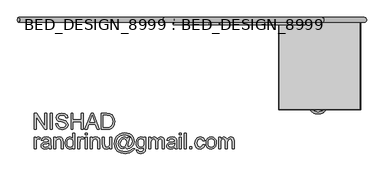
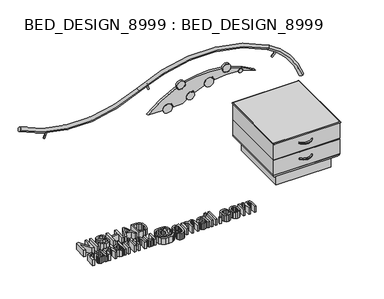
"""IFC4 building model written with IfcOpenShell, lengths in millimetres: furniture geometry, BED_DESIGN_8999 : BED_DESIGN_8999."""

from ifc_helpers import new_model, si_unit, point, frame, frame_2d, origin, origin_with_axes, place, context, project, spatial, polyline, circle_curve, ellipse_curve, trimmed, segment, composite_curve, outline, extrude, source, transform, mapped, element, save
from ifc_brep_helpers import plane_surface, cylinder_surface, revolved_surface, advanced_brep


def bed_design_8999_bed_design_8999_e911dec7(model_context):
    return source(origin(), model_context, "Body", "SolidModel", [
        advanced_brep(
        [(1204.2592917, 1919.1163159, 367.6654044), (1204.2592917, 1919.1163159, 242.6654044), (700.3023182, 1919.1163159, 242.6654044), (700.3023182, 1919.1163159, 367.6654044), (1129.2592917, 1844.1163159, 87.6654044), (1129.2592917, 1844.1163159, 367.6654044), (775.3023182, 1844.1163159, 367.6654044), (775.3023182, 1844.1163159, 87.6654044), (1204.2331329, 1919.0901571, 116.4128697), (1174.2592917, 1889.1163159, 87.6654044), (730.3023182, 1889.1163159, 87.6654044), (700.328477, 1919.0901571, 116.4128697), (1201.7592917, 1916.6163159, 118.9128697), (1201.7592917, 1916.6163159, 116.4128697), (702.8023182, 1916.6163159, 116.4128697), (702.8023182, 1916.6163159, 118.9128697), (1204.2592917, 1919.1163159, 237.6654044), (1204.2592917, 1919.1163159, 118.9128697), (700.3023182, 1919.1163159, 118.9128697), (700.3023182, 1919.1163159, 237.6654044), (1199.2592917, 1914.1163159, 242.6654044), (1199.2592917, 1914.1163159, 237.6654044), (705.3023182, 1914.1163159, 237.6654044), (705.3023182, 1914.1163159, 242.6654044), (700.3023182, 1379.1275792, 242.6654044), (700.3023182, 1379.1275792, 367.6654044), (775.3023182, 1454.1275792, 367.6654044), (775.3023182, 1454.1275792, 87.6654044), (730.3023182, 1409.1275792, 87.6654044), (700.328477, 1379.153738, 116.4128697), (702.8023182, 1381.6275792, 116.4128697), (702.8023182, 1381.6275792, 118.9128697), (700.3023182, 1379.1275792, 118.9128697), (700.3023182, 1379.1275792, 237.6654044), (705.3023182, 1384.1275792, 237.6654044), (705.3023182, 1384.1275792, 242.6654044), (1204.2592917, 1379.1275792, 242.6654044), (1204.2592917, 1379.1275792, 367.6654044), (1129.2592917, 1454.1275792, 367.6654044), (1129.2592917, 1454.1275792, 87.6654044), (1174.2592917, 1409.1275792, 87.6654044), (1204.2331329, 1379.153738, 116.4128697), (1201.7592917, 1381.6275792, 116.4128697), (1201.7592917, 1381.6275792, 118.9128697), (1204.2592917, 1379.1275792, 118.9128697), (1204.2592917, 1379.1275792, 237.6654044), (1199.2592917, 1384.1275792, 237.6654044), (1199.2592917, 1384.1275792, 242.6654044)],
        [
            (0, 1),
            (1, 2),
            (2, 3),
            (3, 0),
            (4, 5),
            (5, 6),
            (6, 7),
            (7, 4),
            (8, 9, ellipse_curve(frame((1174.2592917, 1889.1163159, 117.6654044), z_axis=(-0.7071067811865456, 0.7071067811865496, 0.0), x_axis=(0.7071067811865495, 0.7071067811865455, 0.0)), 42.4264069, 30.0)),
            (9, 10),
            (10, 11, ellipse_curve(frame((730.3023182, 1889.1163159, 117.6654044), z_axis=(0.7071067811865493, 0.7071067811865457, 0.0), x_axis=(0.7071067811865457, -0.7071067811865495, 0.0)), 42.4264069, 30.0)),
            (11, 8),
            (12, 13),
            (13, 14),
            (14, 15),
            (15, 12),
            (16, 17),
            (17, 18),
            (18, 19),
            (19, 16),
            (20, 21),
            (21, 22),
            (22, 23),
            (23, 20),
            (2, 24),
            (24, 25),
            (25, 3),
            (6, 26),
            (26, 27),
            (27, 7),
            (10, 28),
            (28, 29, ellipse_curve(frame((730.3023182, 1409.1275792, 117.6654044), z_axis=(-0.7071067811865457, 0.7071067811865495, 0.0), x_axis=(0.7071067811865495, 0.7071067811865456, 0.0)), 42.4264069, 30.0)),
            (29, 11),
            (14, 30),
            (30, 31),
            (31, 15),
            (18, 32),
            (32, 33),
            (33, 19),
            (22, 34),
            (34, 35),
            (35, 23),
            (24, 36),
            (36, 37),
            (37, 25),
            (26, 38),
            (38, 39),
            (39, 27),
            (28, 40),
            (40, 41, ellipse_curve(frame((1174.2592917, 1409.1275792, 117.6654044), z_axis=(-0.7071067811865496, -0.7071067811865455, 0.0), x_axis=(-0.7071067811865455, 0.7071067811865496, 0.0)), 42.4264069, 30.0)),
            (41, 29),
            (30, 42),
            (42, 43),
            (43, 31),
            (32, 44),
            (44, 45),
            (45, 33),
            (34, 46),
            (46, 47),
            (47, 35),
            (36, 1),
            (0, 37),
            (5, 38),
            (4, 39),
            (9, 40),
            (8, 41),
            (13, 42),
            (12, 43),
            (17, 44),
            (16, 45),
            (21, 46),
            (20, 47),
        ],
        [
            plane_surface(frame((1204.2592917, 1919.1163159, 242.6654044), z_axis=(0.0, 1.0, 0.0), x_axis=(-1.0, 0.0, 0.0))),
            plane_surface(frame((1129.2592917, 1844.1163159, 367.6654044), z_axis=(0.0, -1.0, 0.0), x_axis=(-1.0, 0.0, 0.0))),
            cylinder_surface(frame((1204.2649233, 1889.1163159, 117.6654044), z_axis=(1.0, 0.0, 0.0), x_axis=(0.0, 1.0, 0.0)), 30.0),
            plane_surface(frame((1201.7592917, 1916.6163159, 116.4128697), z_axis=(0.0, 1.0, 0.0), x_axis=(-1.0, 0.0, 0.0))),
            plane_surface(frame((1204.2592917, 1919.1163159, 118.9128697), z_axis=(0.0, 1.0, 0.0), x_axis=(-1.0, 0.0, 0.0))),
            plane_surface(frame((1199.2592917, 1914.1163159, 237.6654044), z_axis=(0.0, 1.0, 0.0), x_axis=(-1.0, 0.0, 0.0))),
            plane_surface(frame((700.3023182, 1919.1163159, 242.6654044), z_axis=(-1.0, 0.0, 0.0), x_axis=(0.0, -1.0, 0.0))),
            plane_surface(frame((775.3023182, 1844.1163159, 367.6654044), z_axis=(1.0, 0.0, 0.0), x_axis=(0.0, -1.0, 0.0))),
            cylinder_surface(frame((730.3023182, 1919.1219475, 117.6654044), z_axis=(0.0, 1.0, 0.0), x_axis=(-1.0, 0.0, 0.0)), 30.0),
            plane_surface(frame((702.8023182, 1916.6163159, 116.4128697), z_axis=(-1.0, 0.0, 0.0), x_axis=(0.0, -1.0, 0.0))),
            plane_surface(frame((700.3023182, 1919.1163159, 118.9128697), z_axis=(-1.0, 0.0, 0.0), x_axis=(0.0, -1.0, 0.0))),
            plane_surface(frame((705.3023182, 1914.1163159, 237.6654044), z_axis=(-1.0, 0.0, 0.0), x_axis=(0.0, -1.0, 0.0))),
            plane_surface(frame((700.3023182, 1379.1275792, 242.6654044), z_axis=(0.0, -1.0, 0.0), x_axis=(1.0, 0.0, 0.0))),
            plane_surface(frame((775.3023182, 1454.1275792, 367.6654044), z_axis=(0.0, 1.0, 0.0), x_axis=(1.0, 0.0, 0.0))),
            cylinder_surface(frame((700.2966866, 1409.1275792, 117.6654044), z_axis=(-1.0, 0.0, 0.0), x_axis=(0.0, -1.0, 0.0)), 30.0),
            plane_surface(frame((702.8023182, 1381.6275792, 116.4128697), z_axis=(0.0, -1.0, 0.0), x_axis=(1.0, 0.0, 0.0))),
            plane_surface(frame((700.3023182, 1379.1275792, 118.9128697), z_axis=(0.0, -1.0, 0.0), x_axis=(1.0, 0.0, 0.0))),
            plane_surface(frame((705.3023182, 1384.1275792, 237.6654044), z_axis=(0.0, -1.0, 0.0), x_axis=(1.0, 0.0, 0.0))),
            plane_surface(frame((1204.2592917, 1379.1275792, 242.6654044), z_axis=(1.0, 0.0, 0.0), x_axis=(0.0, 1.0, 0.0))),
            plane_surface(frame((1204.2592917, 1379.1275792, 367.6654044), z_axis=(0.0, 0.0, 1.0), x_axis=(0.0, 1.0, 0.0))),
            plane_surface(frame((1129.2592917, 1454.1275792, 367.6654044), z_axis=(-1.0, 0.0, 0.0), x_axis=(0.0, 1.0, 0.0))),
            plane_surface(frame((1129.2592917, 1454.1275792, 87.6654044), z_axis=(0.0, 0.0, -1.0), x_axis=(0.0, 1.0, 0.0))),
            cylinder_surface(frame((1174.2592917, 1379.1219475, 117.6654044), z_axis=(0.0, -1.0, 0.0), x_axis=(1.0, 0.0, 0.0)), 30.0),
            plane_surface(frame((1204.2331329, 1379.153738, 116.4128697), z_axis=(0.0, 0.0, 1.0), x_axis=(0.0, 1.0, 0.0))),
            plane_surface(frame((1201.7592917, 1381.6275792, 116.4128697), z_axis=(1.0, 0.0, 0.0), x_axis=(0.0, 1.0, 0.0))),
            plane_surface(frame((1201.7592917, 1381.6275792, 118.9128697), z_axis=(0.0, 0.0, -1.0), x_axis=(0.0, 1.0, 0.0))),
            plane_surface(frame((1204.2592917, 1379.1275792, 118.9128697), z_axis=(1.0, 0.0, 0.0), x_axis=(0.0, 1.0, 0.0))),
            plane_surface(frame((1204.2592917, 1379.1275792, 237.6654044), z_axis=(0.0, 0.0, 1.0), x_axis=(0.0, 1.0, 0.0))),
            plane_surface(frame((1199.2592917, 1384.1275792, 237.6654044), z_axis=(1.0, 0.0, 0.0), x_axis=(0.0, 1.0, 0.0))),
            plane_surface(frame((1199.2592917, 1384.1275792, 242.6654044), z_axis=(0.0, 0.0, -1.0), x_axis=(0.0, 1.0, 0.0))),
        ],
        [
            (0, [[1, 2, 3, 4]]),
            (1, [[5, 6, 7, 8]]),
            (2, [[9, 10, 11, 12]]),
            (3, [[13, 14, 15, 16]]),
            (4, [[17, 18, 19, 20]]),
            (5, [[21, 22, 23, 24]]),
            (6, [[-3, 25, 26, 27]]),
            (7, [[-7, 28, 29, 30]]),
            (8, [[-11, 31, 32, 33]]),
            (9, [[-15, 34, 35, 36]]),
            (10, [[-19, 37, 38, 39]]),
            (11, [[-23, 40, 41, 42]]),
            (12, [[-26, 43, 44, 45]]),
            (13, [[-29, 46, 47, 48]]),
            (14, [[-32, 49, 50, 51]]),
            (15, [[-35, 52, 53, 54]]),
            (16, [[-38, 55, 56, 57]]),
            (17, [[-41, 58, 59, 60]]),
            (18, [[-44, 61, -1, 62]]),
            (19, [[-27, -45, -62, -4], [63, -46, -28, -6]]),
            (20, [[-47, -63, -5, 64]]),
            (21, [[65, -49, -31, -10], [-30, -48, -64, -8]]),
            (22, [[-50, -65, -9, 66]]),
            (23, [[-33, -51, -66, -12], [67, -52, -34, -14]]),
            (24, [[-53, -67, -13, 68]]),
            (25, [[69, -55, -37, -18], [-36, -54, -68, -16]]),
            (26, [[-56, -69, -17, 70]]),
            (27, [[-39, -57, -70, -20], [71, -58, -40, -22]]),
            (28, [[-59, -71, -21, 72]]),
            (29, [[-61, -43, -25, -2], [-42, -60, -72, -24]]),
        ],
    ),
        extrude(outline(polyline([(1204.2592917, 1919.1163159), (1204.2592917, 1379.1275792), (700.3023182, 1379.1275792), (700.3023182, 1919.1163159), (1204.2592917, 1919.1163159)])), frame((0.0, 0.0, 367.6654044), z_axis=(0.0, 0.0, 1.0), x_axis=(1.0, 0.0, 0.0)), (0.0, 0.0, 1.0), 10.0),
        advanced_brep(
        [(1204.2592917, 1919.8890651, 377.6654044), (1204.2592917, 1919.8890651, 367.6654044), (704.2592917, 1919.8890651, 367.6654044), (704.2592917, 1919.8890651, 377.6654044), (704.2592917, 1379.8890651, 367.6654044), (704.2592917, 1379.8890651, 377.6654044), (1204.2592917, 1379.8890651, 367.6654044), (1204.2592917, 1379.8890651, 377.6654044)],
        [
            (0, 1, ellipse_curve(frame((1204.2592917, 1919.8890651, 372.6654044), z_axis=(-0.7071067811865456, 0.7071067811865496, 0.0), x_axis=(0.7071067811865493, 0.7071067811865456, 0.0)), 7.0710678, 5.0)),
            (1, 2),
            (2, 3, ellipse_curve(frame((704.2592917, 1919.8890651, 372.6654044), z_axis=(0.7071067811865496, 0.7071067811865456, 0.0), x_axis=(0.7071067811865454, -0.7071067811865496, 0.0)), 7.0710678, 5.0)),
            (3, 0),
            (1, 0),
            (3, 2),
            (2, 4),
            (4, 5, ellipse_curve(frame((704.2592917, 1379.8890651, 372.6654044), z_axis=(-0.7071067811865454, 0.7071067811865496, 0.0), x_axis=(0.7071067811865495, 0.7071067811865456, 0.0)), 7.0710678, 5.0)),
            (5, 3),
            (5, 4),
            (4, 6),
            (6, 7, ellipse_curve(frame((1204.2592917, 1379.8890651, 372.6654044), z_axis=(-0.7071067811865496, -0.7071067811865454, 0.0), x_axis=(-0.7071067811865456, 0.7071067811865495, 0.0)), 7.0710678, 5.0)),
            (7, 5),
            (7, 6),
            (6, 1),
            (0, 7),
        ],
        [
            cylinder_surface(frame((1204.2592917, 1919.8890651, 372.6654044), z_axis=(1.0, 0.0, 0.0), x_axis=(0.0, 1.0, 0.0)), 5.0),
            plane_surface(frame((1204.2592917, 1919.8890651, 377.6654044), z_axis=(0.0, -1.0, 0.0), x_axis=(-1.0, 0.0, 0.0))),
            cylinder_surface(frame((704.2592917, 1919.8890651, 372.6654044), z_axis=(0.0, 1.0, 0.0), x_axis=(-1.0, 0.0, 0.0)), 5.0),
            plane_surface(frame((704.2592917, 1919.8890651, 377.6654044), z_axis=(1.0, 0.0, 0.0), x_axis=(0.0, -1.0, 0.0))),
            cylinder_surface(frame((704.2592917, 1379.8890651, 372.6654044), z_axis=(-1.0, 0.0, 0.0), x_axis=(0.0, -1.0, 0.0)), 5.0),
            plane_surface(frame((704.2592917, 1379.8890651, 377.6654044), z_axis=(0.0, 1.0, 0.0), x_axis=(1.0, 0.0, 0.0))),
            cylinder_surface(frame((1204.2592917, 1379.8890651, 372.6654044), z_axis=(0.0, -1.0, 0.0), x_axis=(1.0, 0.0, 0.0)), 5.0),
            plane_surface(frame((1204.2592917, 1379.8890651, 377.6654044), z_axis=(-1.0, 0.0, 0.0), x_axis=(0.0, 1.0, 0.0))),
        ],
        [
            (0, [[1, 2, 3, 4]]),
            (1, [[5, -4, 6, -2]]),
            (2, [[-3, 7, 8, 9]]),
            (3, [[-6, -9, 10, -7]]),
            (4, [[-8, 11, 12, 13]]),
            (5, [[-10, -13, 14, -11]]),
            (6, [[-12, 15, -1, 16]]),
            (7, [[-14, -16, -5, -15]]),
        ],
    ),
        extrude(outline(polyline([(1163.4030291, 1880.0), (1163.4030291, 1422.837799), (744.2592917, 1422.837799), (744.2592917, 1880.0), (1163.4030291, 1880.0)])), origin_with_axes(), (0.0, 0.0, 1.0), 150.0),
        advanced_brep(
        [(899.6687999, 1386.6145304, 185.0), (890.9935307, 1381.640628, 185.0), (990.9935307, 1386.6145304, 185.0), (999.6687999, 1381.640628, 185.0)],
        [
            (0, 1, circle_curve(frame((895.3311653, 1384.1275792, 185.0), z_axis=(-0.4973902333108333, 0.8675269193558173, 0.0), x_axis=(-0.8675269193558173, -0.4973902333108333, 0.0)), 5.0)),
            (1, 0, circle_curve(frame((895.3311653, 1384.1275792, 185.0), z_axis=(-0.4973902333108333, 0.8675269193558173, 0.0), x_axis=(-0.8675269193558173, -0.4973902333108333, 0.0)), 5.0)),
            (2, 3, circle_curve(frame((995.3311653, 1384.1275792, 185.0), z_axis=(0.49739023331085336, 0.867526919355806, 0.0), x_axis=(0.867526919355806, -0.49739023331085336, 0.0)), 5.0)),
            (3, 2, circle_curve(frame((995.3311653, 1384.1275792, 185.0), z_axis=(0.49739023331085336, 0.867526919355806, 0.0), x_axis=(0.867526919355806, -0.49739023331085336, 0.0)), 5.0)),
            (3, 1, circle_curve(frame((945.3311653, 1412.7947146, 185.0), z_axis=(0.0, 0.0, -1.0), x_axis=(-0.8675269193558204, -0.497390233310828, 0.0)), 62.6350991)),
            (0, 2, circle_curve(frame((945.3311653, 1412.7947146, 185.0), z_axis=(0.0, 0.0, 1.0), x_axis=(-0.8675269193558204, -0.497390233310828, 0.0)), 52.6350991)),
        ],
        [
            plane_surface(frame((895.3311653, 1384.1275792, 0.0), z_axis=(-0.497390233310828, 0.8675269193558204, 0.0), x_axis=(0.0, 0.0, 1.0))),
            plane_surface(frame((995.3311653, 1384.1275792, 0.0), z_axis=(0.49739023331085874, 0.8675269193558027, 0.0), x_axis=(0.0, 0.0, 1.0))),
            revolved_surface(trimmed(ellipse_curve(frame((895.3311653, 1384.1275792, 185.0), z_axis=(-0.4973902333108333, 0.8675269193558173, 0.0), x_axis=(-0.8675269193558173, -0.4973902333108333, 0.0)), 5.0, 5.0), [point((899.6687999, 1386.6145304, 185.0))], [point((890.9935307, 1381.640628, 185.0))], True, "CARTESIAN"), (945.3311653, 1412.7947146, 0.0), (0.0, 0.0, 1.0)),
            revolved_surface(trimmed(ellipse_curve(frame((895.3311653, 1384.1275792, 185.0), z_axis=(-0.4973902333108333, 0.8675269193558173, 0.0), x_axis=(-0.8675269193558173, -0.4973902333108333, 0.0)), 5.0, 5.0), [point((890.9935307, 1381.640628, 185.0))], [point((899.6687999, 1386.6145304, 185.0))], True, "CARTESIAN"), (945.3311653, 1412.7947146, 0.0), (0.0, 0.0, 1.0)),
        ],
        [
            (0, [[1, 2]]),
            (1, [[3, 4]]),
            (2, [[5, -1, 6, -4]]),
            (3, [[-6, -2, -5, -3]]),
        ],
    ),
        advanced_brep(
        [(899.6687999, 1386.6145304, 311.8762673), (890.9935307, 1381.640628, 311.8762673), (990.9935307, 1386.6145304, 311.8762673), (999.6687999, 1381.640628, 311.8762673)],
        [
            (0, 1, circle_curve(frame((895.3311653, 1384.1275792, 311.8762673), z_axis=(-0.4973902333108333, 0.8675269193558173, 0.0), x_axis=(-0.8675269193558173, -0.4973902333108333, 0.0)), 5.0)),
            (1, 0, circle_curve(frame((895.3311653, 1384.1275792, 311.8762673), z_axis=(-0.4973902333108333, 0.8675269193558173, 0.0), x_axis=(-0.8675269193558173, -0.4973902333108333, 0.0)), 5.0)),
            (2, 3, circle_curve(frame((995.3311653, 1384.1275792, 311.8762673), z_axis=(0.49739023331085336, 0.867526919355806, 0.0), x_axis=(0.867526919355806, -0.49739023331085336, 0.0)), 5.0)),
            (3, 2, circle_curve(frame((995.3311653, 1384.1275792, 311.8762673), z_axis=(0.49739023331085336, 0.867526919355806, 0.0), x_axis=(0.867526919355806, -0.49739023331085336, 0.0)), 5.0)),
            (3, 1, circle_curve(frame((945.3311653, 1412.7947146, 311.8762673), z_axis=(0.0, 0.0, -1.0), x_axis=(-0.8675269193558204, -0.497390233310828, 0.0)), 62.6350991)),
            (0, 2, circle_curve(frame((945.3311653, 1412.7947146, 311.8762673), z_axis=(0.0, 0.0, 1.0), x_axis=(-0.8675269193558204, -0.497390233310828, 0.0)), 52.6350991)),
        ],
        [
            plane_surface(frame((895.3311653, 1384.1275792, 126.8762673), z_axis=(-0.497390233310828, 0.8675269193558204, 0.0), x_axis=(0.0, 0.0, 1.0))),
            plane_surface(frame((995.3311653, 1384.1275792, 126.8762673), z_axis=(0.49739023331085874, 0.8675269193558027, 0.0), x_axis=(0.0, 0.0, 1.0))),
            revolved_surface(trimmed(ellipse_curve(frame((895.3311653, 1384.1275792, 311.8762673), z_axis=(-0.4973902333108333, 0.8675269193558173, 0.0), x_axis=(-0.8675269193558173, -0.4973902333108333, 0.0)), 5.0, 5.0), [point((899.6687999, 1386.6145304, 311.8762673))], [point((890.9935307, 1381.640628, 311.8762673))], True, "CARTESIAN"), (945.3311653, 1412.7947146, 126.8762673), (0.0, 0.0, 1.0)),
            revolved_surface(trimmed(ellipse_curve(frame((895.3311653, 1384.1275792, 311.8762673), z_axis=(-0.4973902333108333, 0.8675269193558173, 0.0), x_axis=(-0.8675269193558173, -0.4973902333108333, 0.0)), 5.0, 5.0), [point((890.9935307, 1381.640628, 311.8762673))], [point((899.6687999, 1386.6145304, 311.8762673))], True, "CARTESIAN"), (945.3311653, 1412.7947146, 126.8762673), (0.0, 0.0, 1.0)),
        ],
        [
            (0, [[1, 2]]),
            (1, [[3, 4]]),
            (2, [[5, -1, 6, -4]]),
            (3, [[-6, -2, -5, -3]]),
        ],
    ),
        advanced_brep(
        [(-917.2940752, 1950.0, 720.0997199), (-917.2940752, 1920.0, 720.0997199), (-14.3645373, 1920.0, 720.0997199), (-14.3645373, 1950.0, 720.0997199), (974.3645373, 1920.0, 720.0997199), (974.3645373, 1950.0, 720.0997199), (1232.6909698, 1950.0, 412.2382658), (1232.6909698, 1920.0, 412.2382658)],
        [
            (0, 1, circle_curve(frame((-917.2940752, 1935.0, 720.0997199), z_axis=(-0.8779142380210138, 0.0, 0.47881790973185484), x_axis=(0.0, -1.0, 0.0)), 15.0)),
            (1, 0, circle_curve(frame((-917.2940752, 1935.0, 720.0997199), z_axis=(-0.8779142380210138, 0.0, 0.47881790973185484), x_axis=(0.0, -1.0, 0.0)), 15.0)),
            (2, 1, circle_curve(frame((-465.8293063, 1920.0, 1547.8618829), z_axis=(0.0, 1.0, 0.0), x_axis=(-0.47881790973187277, 0.0, -0.877914238021004)), 942.8736056)),
            (0, 3, circle_curve(frame((-465.8293063, 1950.0, 1547.8618829), z_axis=(0.0, -1.0, 0.0), x_axis=(-0.47881790973187277, 0.0, -0.877914238021004)), 942.8736056)),
            (3, 2, circle_curve(frame((-14.3645373, 1935.0, 720.0997199), z_axis=(-0.8779142380210219, 0.0, -0.4788179097318398), x_axis=(0.0, -1.0, 0.0)), 15.0)),
            (2, 3, circle_curve(frame((-14.3645373, 1935.0, 720.0997199), z_axis=(-0.8779142380210219, 0.0, -0.4788179097318398), x_axis=(0.0, -1.0, 0.0)), 15.0)),
            (4, 2, circle_curve(frame((480.0, 1920.0, -186.3193117), z_axis=(0.0, -1.0, 0.0), x_axis=(-0.4788179097318431, 0.0, 0.8779142380210202)), 1032.4687679)),
            (3, 5, circle_curve(frame((480.0, 1950.0, -186.3193117), z_axis=(0.0, 1.0, 0.0), x_axis=(-0.4788179097318431, 0.0, 0.8779142380210202)), 1032.4687679)),
            (5, 4, circle_curve(frame((974.3645373, 1935.0, 720.0997199), z_axis=(-0.8779142380210557, 0.0, 0.47881790973177796), x_axis=(0.0, -1.0, 0.0)), 15.0)),
            (4, 5, circle_curve(frame((974.3645373, 1935.0, 720.0997199), z_axis=(-0.8779142380210557, 0.0, 0.47881790973177796), x_axis=(0.0, -1.0, 0.0)), 15.0)),
            (6, 7, circle_curve(frame((1232.6909698, 1935.0, 412.2382658), z_axis=(0.31909538220484907, 0.0, -0.9477226055421182), x_axis=(0.0, -1.0, 0.0)), 15.0)),
            (7, 6, circle_curve(frame((1232.6909698, 1935.0, 412.2382658), z_axis=(0.31909538220484907, 0.0, -0.9477226055421182), x_axis=(0.0, -1.0, 0.0)), 15.0)),
            (7, 4, circle_curve(frame((710.5767707, 1920.0, 236.443968), z_axis=(0.0, -1.0, 0.0), x_axis=(0.4788179097317882, 0.0, 0.8779142380210502)), 550.9145779)),
            (5, 6, circle_curve(frame((710.5767707, 1950.0, 236.443968), z_axis=(0.0, 1.0, 0.0), x_axis=(0.4788179097317882, 0.0, 0.8779142380210502)), 550.9145779)),
        ],
        [
            plane_surface(frame((-917.2940752, 0.0, 720.0997199), z_axis=(-0.8779142380210041, 0.0, 0.4788179097318728), x_axis=(0.0, -1.0, 0.0))),
            revolved_surface(trimmed(ellipse_curve(frame((-917.2940752, 1935.0, 720.0997199), z_axis=(-0.8779142380210138, 0.0, 0.47881790973185484), x_axis=(0.0, -1.0, 0.0)), 15.0, 15.0), [point((-917.2940752, 1950.0, 720.0997199))], [point((-917.2940752, 1920.0, 720.0997199))], True, "CARTESIAN"), (-465.8293063, 0.0, 1547.8618829), (0.0, -1.0, 0.0)),
            revolved_surface(trimmed(ellipse_curve(frame((-917.2940752, 1935.0, 720.0997199), z_axis=(-0.8779142380210138, 0.0, 0.47881790973185484), x_axis=(0.0, -1.0, 0.0)), 15.0, 15.0), [point((-917.2940752, 1920.0, 720.0997199))], [point((-917.2940752, 1950.0, 720.0997199))], True, "CARTESIAN"), (-465.8293063, 0.0, 1547.8618829), (0.0, -1.0, 0.0)),
            revolved_surface(trimmed(ellipse_curve(frame((-14.3645373, 1935.0, 720.0997199), z_axis=(-0.8779142380210104, 0.0, -0.47881790973186106), x_axis=(0.0, -1.0, 0.0)), 15.0, 15.0), [point((-14.3645373, 1950.0, 720.0997199))], [point((-14.3645373, 1920.0, 720.0997199))], True, "CARTESIAN"), (480.0, 0.0, -186.3193117), (0.0, 1.0, 0.0)),
            revolved_surface(trimmed(ellipse_curve(frame((-14.3645373, 1935.0, 720.0997199), z_axis=(-0.8779142380210104, 0.0, -0.47881790973186106), x_axis=(0.0, -1.0, 0.0)), 15.0, 15.0), [point((-14.3645373, 1920.0, 720.0997199))], [point((-14.3645373, 1950.0, 720.0997199))], True, "CARTESIAN"), (480.0, 0.0, -186.3193117), (0.0, 1.0, 0.0)),
            plane_surface(frame((1232.6909698, 0.0, 412.2382658), z_axis=(0.31909538220482964, 0.0, -0.9477226055421247), x_axis=(0.0, -1.0, 0.0))),
            revolved_surface(trimmed(ellipse_curve(frame((974.3645373, 1935.0, 720.0997199), z_axis=(-0.87791423802106, 0.0, 0.47881790973177024), x_axis=(0.0, -1.0, 0.0)), 15.0, 15.0), [point((974.3645373, 1950.0, 720.0997199))], [point((974.3645373, 1920.0, 720.0997199))], True, "CARTESIAN"), (710.5767707, 0.0, 236.443968), (0.0, 1.0, 0.0)),
            revolved_surface(trimmed(ellipse_curve(frame((974.3645373, 1935.0, 720.0997199), z_axis=(-0.87791423802106, 0.0, 0.47881790973177024), x_axis=(0.0, -1.0, 0.0)), 15.0, 15.0), [point((974.3645373, 1920.0, 720.0997199))], [point((974.3645373, 1950.0, 720.0997199))], True, "CARTESIAN"), (710.5767707, 0.0, 236.443968), (0.0, 1.0, 0.0)),
        ],
        [
            (0, [[1, 2]]),
            (1, [[3, -1, 4, 5]]),
            (2, [[-4, -2, -3, 6]]),
            (3, [[7, -5, 8, 9]]),
            (4, [[-8, -6, -7, 10]]),
            (5, [[11, 12]]),
            (6, [[13, -9, 14, -12]]),
            (7, [[-14, -10, -13, -11]]),
        ],
    ),
        extrude(outline(composite_curve([segment(trimmed(circle_curve(frame_2d((0.0, -5.0)), 5.0), [point((0.0, -10.0))], [point((0.0, 0.0))], False, "CARTESIAN"), True, "CONTINUOUS"), segment(trimmed(circle_curve(frame_2d((0.0, -5.0)), 5.0), [point((0.0, 0.0))], [point((0.0, -10.0))], False, "CARTESIAN"), True, "CONTINUOUS")], self_intersect=False)), frame((-724.5433295, 1935.7468402, 579.9741393), z_axis=(0.3090169943749533, 0.0, 0.9510565162951516), x_axis=(0.0, -1.0, 0.0)), (0.0, 0.0, 1.0), 52.5099877),
        extrude(outline(composite_curve([segment(trimmed(circle_curve(frame_2d((0.0, -4.9999999)), 5.0), [point((0.0, -10.0))], [point((0.0, 0.0))], False, "CARTESIAN"), True, "CONTINUOUS"), segment(trimmed(circle_curve(frame_2d((0.0, -4.9999999)), 5.0), [point((0.0, 0.0))], [point((0.0, -10.0))], False, "CARTESIAN"), True, "CONTINUOUS")], self_intersect=False)), frame((61.28639, 1935.7468402, 700.2448457), z_axis=(-0.30901699437495017, 0.0, 0.9510565162951528), x_axis=(0.0, 1.0, 0.0)), (0.0, 0.0, 1.0), 52.5099877),
        extrude(outline(composite_curve([segment(trimmed(circle_curve(frame_2d((0.0, -5.0)), 5.0), [point((0.0, -10.0))], [point((0.0, 0.0))], False, "CARTESIAN"), True, "CONTINUOUS"), segment(trimmed(circle_curve(frame_2d((0.0, -5.0)), 5.0), [point((0.0, 0.0))], [point((0.0, -10.0))], False, "CARTESIAN"), True, "CONTINUOUS")], self_intersect=False)), frame((1010.7295294, 1935.7468402, 629.3857141), z_axis=(0.7089330900730306, 0.0, 0.7052757430959214), x_axis=(0.0, -1.0, 0.0)), (0.0, 0.0, 1.0), 52.5099877),
        extrude(outline(composite_curve([segment(trimmed(circle_curve(frame_2d((51.784971, 501.9071903)), 651.327435), [point((658.3434442, 264.6009618))], [point((515.2024865, 44.2264786))], False, "CARTESIAN"), True, "CONTINUOUS"), segment(polyline([(515.2024865, 44.2264786), (515.2024865, 155.9954837)]), True, "CONTINUOUS"), segment(trimmed(circle_curve(frame_2d((515.2024865, 195.9954837)), 40.0), [point((515.2024865, 155.9954837))], [point((515.2024865, 235.9954837))], True, "CARTESIAN"), True, "CONTINUOUS"), segment(polyline([(515.2024865, 235.9954837), (515.2024865, 309.5211021)]), True, "CONTINUOUS"), segment(trimmed(circle_curve(frame_2d((86.9183012, 652.4642393)), 548.6686967), [point((515.2024865, 309.5211021))], [point((538.2621217, 340.4929354))], True, "CARTESIAN"), True, "CONTINUOUS"), segment(trimmed(circle_curve(frame_2d((557.2345685, 369.9046042)), 35.0), [point((538.2621217, 340.4929354))], [point((574.293175, 400.4660823))], True, "CARTESIAN"), True, "CONTINUOUS"), segment(trimmed(circle_curve(frame_2d((86.9183012, 652.4642393)), 548.6686967), [point((574.293175, 400.4660823))], [point((605.6663736, 473.7528068))], True, "CARTESIAN"), True, "CONTINUOUS"), segment(trimmed(circle_curve(frame_2d((617.3078852, 512.0212691)), 40.0), [point((605.6663736, 473.7528068))], [point((626.1303999, 551.0361795))], True, "CARTESIAN"), True, "CONTINUOUS"), segment(trimmed(circle_curve(frame_2d((86.9183012, 652.4642393)), 548.6686967), [point((626.1303999, 551.0361795))], [point((629.98055, 730.6993505))], True, "CARTESIAN"), True, "CONTINUOUS"), segment(trimmed(circle_curve(frame_2d((626.7684137, 750.4397198)), 20.0), [point((629.98055, 730.6993505))], [point((622.8389575, 770.0499052))], True, "CARTESIAN"), True, "CONTINUOUS"), segment(trimmed(circle_curve(frame_2d((86.9183012, 652.4642393)), 548.6686967), [point((622.8389575, 770.0499052))], [point((593.139423, 864.0712206))], True, "CARTESIAN"), True, "CONTINUOUS"), segment(trimmed(circle_curve(frame_2d((51.784971, 501.9071903)), 651.327435), [point((593.139423, 864.0712206))], [point((678.4843614, 679.3199904))], False, "CARTESIAN"), True, "CONTINUOUS"), segment(trimmed(circle_curve(frame_2d((687.1096179, 645.3994222)), 35.0), [point((678.4843614, 679.3199904))], [point((693.9003096, 611.0645055))], True, "CARTESIAN"), True, "CONTINUOUS"), segment(trimmed(circle_curve(frame_2d((51.784971, 501.9071903)), 651.327435), [point((693.9003096, 611.0645055))], [point((680.3009283, 331.0413981))], False, "CARTESIAN"), True, "CONTINUOUS"), segment(trimmed(circle_curve(frame_2d((670.2150763, 297.5260943)), 35.0), [point((680.3009283, 331.0413981))], [point((658.3434442, 264.6009618))], True, "CARTESIAN"), True, "CONTINUOUS")], self_intersect=False)), frame((0.0, 1904.8168466, 0.0), z_axis=(0.0, 1.0, 0.0), x_axis=(0.0, 0.0, 1.0)), (0.0, 0.0, 1.0), 15.0722185),
        extrude(outline(composite_curve([segment(trimmed(circle_curve(frame_2d((670.2150763, 297.5260943)), 30.0), [point((670.2150763, 267.5260943))], [point((670.2150763, 327.5260943))], False, "CARTESIAN"), True, "CONTINUOUS"), segment(trimmed(circle_curve(frame_2d((670.2150763, 297.5260943)), 30.0), [point((670.2150763, 327.5260943))], [point((670.2150763, 267.5260943))], False, "CARTESIAN"), True, "CONTINUOUS")], self_intersect=False)), frame((0.0, 1904.8168466, 0.0), z_axis=(0.0, 1.0, 0.0), x_axis=(0.0, 0.0, 1.0)), (0.0, 0.0, 1.0), 15.0722185),
        extrude(outline(composite_curve([segment(trimmed(circle_curve(frame_2d((617.3078852, 512.0212691)), 35.0), [point((617.3078852, 477.0212691))], [point((617.3078852, 547.0212691))], False, "CARTESIAN"), True, "CONTINUOUS"), segment(trimmed(circle_curve(frame_2d((617.3078852, 512.0212691)), 35.0), [point((617.3078852, 547.0212691))], [point((617.3078852, 477.0212691))], False, "CARTESIAN"), True, "CONTINUOUS")], self_intersect=False)), frame((0.0, 1904.8168466, 0.0), z_axis=(0.0, 1.0, 0.0), x_axis=(0.0, 0.0, 1.0)), (0.0, 0.0, 1.0), 15.0722185),
        extrude(outline(composite_curve([segment(trimmed(circle_curve(frame_2d((515.2024865, 195.9954837)), 35.0), [point((515.2024865, 160.9954837))], [point((515.2024865, 230.9954837))], False, "CARTESIAN"), True, "CONTINUOUS"), segment(trimmed(circle_curve(frame_2d((515.2024865, 195.9954837)), 35.0), [point((515.2024865, 230.9954837))], [point((515.2024865, 160.9954837))], False, "CARTESIAN"), True, "CONTINUOUS")], self_intersect=False)), frame((0.0, 1904.8168466, 0.0), z_axis=(0.0, 1.0, 0.0), x_axis=(0.0, 0.0, 1.0)), (0.0, 0.0, 1.0), 15.0722185),
        extrude(outline(composite_curve([segment(trimmed(circle_curve(frame_2d((687.1096179, 645.3994222)), 30.0), [point((687.1096179, 615.3994222))], [point((687.1096179, 675.3994222))], False, "CARTESIAN"), True, "CONTINUOUS"), segment(trimmed(circle_curve(frame_2d((687.1096179, 645.3994222)), 30.0), [point((687.1096179, 675.3994222))], [point((687.1096179, 615.3994222))], False, "CARTESIAN"), True, "CONTINUOUS")], self_intersect=False)), frame((0.0, 1904.8168466, 0.0), z_axis=(0.0, 1.0, 0.0), x_axis=(0.0, 0.0, 1.0)), (0.0, 0.0, 1.0), 15.0722185),
        extrude(outline(composite_curve([segment(trimmed(circle_curve(frame_2d((626.7684137, 750.4397198)), 15.0), [point((626.7684137, 735.4397198))], [point((626.7684137, 765.4397198))], False, "CARTESIAN"), True, "CONTINUOUS"), segment(trimmed(circle_curve(frame_2d((626.7684137, 750.4397198)), 15.0), [point((626.7684137, 765.4397198))], [point((626.7684137, 735.4397198))], False, "CARTESIAN"), True, "CONTINUOUS")], self_intersect=False)), frame((0.0, 1904.8168466, 0.0), z_axis=(0.0, 1.0, 0.0), x_axis=(0.0, 0.0, 1.0)), (0.0, 0.0, 1.0), 15.0722185),
        extrude(outline(composite_curve([segment(trimmed(circle_curve(frame_2d((557.2345685, 369.9046042)), 30.0), [point((557.2345685, 339.9046042))], [point((557.2345685, 399.9046042))], False, "CARTESIAN"), True, "CONTINUOUS"), segment(trimmed(circle_curve(frame_2d((557.2345685, 369.9046042)), 30.0), [point((557.2345685, 399.9046042))], [point((557.2345685, 339.9046042))], False, "CARTESIAN"), True, "CONTINUOUS")], self_intersect=False)), frame((0.0, 1904.8168466, 0.0), z_axis=(0.0, 1.0, 0.0), x_axis=(0.0, 0.0, 1.0)), (0.0, 0.0, 1.0), 15.0722185),
        extrude(outline(polyline([(-819.039193, 1254.4987071), (-819.039193, 1352.9602456), (-805.8661161, 1352.9602456), (-754.4238084, 1274.9554379), (-754.4238084, 1352.9602456), (-742.1161161, 1352.9602456), (-742.1161161, 1254.4987071), (-755.289193, 1254.4987071), (-806.7315007, 1332.5275533), (-806.7315007, 1254.4987071), (-819.039193, 1254.4987071)])), frame((0.0, 0.0, 70.0), z_axis=(0.0, 0.0, 1.0), x_axis=(1.0, 0.0, 0.0)), (0.0, 0.0, 1.0), 50.0),
        extrude(outline(polyline([(-719.039193, 1254.4987071), (-719.039193, 1352.9602456), (-706.7315007, 1352.9602456), (-706.7315007, 1254.4987071), (-719.039193, 1254.4987071)])), frame((0.0, 0.0, 70.0), z_axis=(0.0, 0.0, 1.0), x_axis=(1.0, 0.0, 0.0)), (0.0, 0.0, 1.0), 50.0),
        extrude(outline(polyline([(-686.7315007, 1288.344861), (-674.4238084, 1288.344861), (-670.4574622, 1276.0251495), (-660.7699622, 1268.2366879), (-646.0103468, 1265.2679379), (-633.1497699, 1267.5155341), (-624.8444814, 1273.6934187), (-622.1161161, 1281.9506302), (-624.1593853, 1289.6309187), (-632.5247699, 1295.219861), (-650.445443, 1299.9193802), (-669.7363084, 1305.9890918), (-680.2050584, 1315.1477456), (-683.6545776, 1327.3833225), (-679.3877507, 1341.313611), (-666.9238084, 1351.1453418), (-648.6786161, 1354.4987071), (-629.2074622, 1350.9890918), (-616.226693, 1340.6765918), (-611.3468853, 1325.2679379), (-623.6545776, 1325.2679379), (-630.6257314, 1337.9121687), (-648.1978468, 1342.1910148), (-665.8180391, 1337.9602456), (-671.3468853, 1327.7438995), (-667.4286161, 1319.2102456), (-647.3324622, 1312.3352456), (-625.5536161, 1306.157361), (-613.6425584, 1296.1813995), (-609.8084237, 1282.2631302), (-614.2194814, 1267.5395725), (-626.9117891, 1256.7943802), (-645.5295776, 1252.9602456), (-667.5127507, 1257.094861), (-681.4190007, 1269.5467841), (-686.7315007, 1288.344861)])), frame((0.0, 0.0, 70.0), z_axis=(0.0, 0.0, 1.0), x_axis=(1.0, 0.0, 0.0)), (0.0, 0.0, 1.0), 50.0),
        extrude(outline(polyline([(-591.3468853, 1254.4987071), (-591.3468853, 1352.9602456), (-579.039193, 1352.9602456), (-579.039193, 1312.9602456), (-526.7315007, 1312.9602456), (-526.7315007, 1352.9602456), (-514.4238084, 1352.9602456), (-514.4238084, 1254.4987071), (-526.7315007, 1254.4987071), (-526.7315007, 1300.6525533), (-579.039193, 1300.6525533), (-579.039193, 1254.4987071), (-591.3468853, 1254.4987071)])), frame((0.0, 0.0, 70.0), z_axis=(0.0, 0.0, 1.0), x_axis=(1.0, 0.0, 0.0)), (0.0, 0.0, 1.0), 50.0),
        extrude(outline(polyline([(-504.3276545, 1254.4987071), (-465.0247699, 1352.9602456), (-454.5440007, 1352.9602456), (-415.2651545, 1254.4987071), (-428.2699622, 1254.4987071), (-439.5199622, 1285.2679379), (-480.0968853, 1285.2679379), (-491.3468853, 1254.4987071), (-504.3276545, 1254.4987071)]), holes=[polyline([(-475.5776545, 1297.5756302), (-444.0151545, 1297.5756302), (-452.9093853, 1321.782361), (-459.8084237, 1340.6525533), (-465.9382314, 1323.8977456), (-475.5776545, 1297.5756302)])]), frame((0.0, 0.0, 70.0), z_axis=(0.0, 0.0, 1.0), x_axis=(1.0, 0.0, 0.0)), (0.0, 0.0, 1.0), 50.0),
        extrude(outline(polyline([(-402.1161161, 1254.4987071), (-402.1161161, 1352.9602456), (-368.1497699, 1352.9602456), (-350.5776545, 1351.5419764), (-336.1065007, 1344.4987071), (-324.4478468, 1327.6717841), (-320.5776545, 1304.2583225), (-323.1978468, 1284.3905341), (-329.9286161, 1270.0515918), (-338.9190007, 1261.1213033), (-350.6858276, 1256.1813995), (-366.5151545, 1254.4987071), (-402.1161161, 1254.4987071)]), holes=[polyline([(-389.8084237, 1266.8063995), (-368.0295776, 1266.8063995), (-352.1882314, 1268.5852456), (-343.0536161, 1273.6092841), (-335.5656353, 1285.8328418), (-332.8853468, 1304.4506302), (-334.1984478, 1317.8640918), (-338.1377507, 1327.7679379), (-350.914193, 1338.6813995), (-368.3661161, 1340.6525533), (-389.8084237, 1340.6525533), (-389.8084237, 1266.8063995)])]), frame((0.0, 0.0, 70.0), z_axis=(0.0, 0.0, 1.0), x_axis=(1.0, 0.0, 0.0)), (0.0, 0.0, 1.0), 50.0),
        extrude(outline(polyline([(-820.5776545, 1132.9602456), (-820.5776545, 1205.2679379), (-809.8084237, 1205.2679379), (-809.8084237, 1194.5708225), (-802.164193, 1204.4265918), (-794.4718853, 1206.8063995), (-782.1161161, 1203.0083225), (-786.226693, 1191.9746687), (-794.8805391, 1194.4987071), (-801.8396737, 1192.0708225), (-806.2747699, 1185.3400533), (-808.2699622, 1170.9650533), (-808.2699622, 1132.9602456), (-820.5776545, 1132.9602456)])), frame((0.0, 0.0, 70.0), z_axis=(0.0, 0.0, 1.0), x_axis=(1.0, 0.0, 0.0)), (0.0, 0.0, 1.0), 50.0),
        extrude(outline(polyline([(-728.2699622, 1142.1910148), (-740.2050584, 1133.8496687), (-753.3901545, 1131.4217841), (-763.6756112, 1132.8821206), (-771.2627507, 1137.2631302), (-775.9412362, 1143.9157745), (-777.5007314, 1152.1910148), (-775.1449622, 1161.9265918), (-768.9550584, 1168.9938995), (-760.3372699, 1173.032361), (-749.6882314, 1174.8833225), (-728.3420776, 1179.1140918), (-728.2699622, 1181.8544764), (-731.6593853, 1190.9410148), (-745.2651545, 1194.4987071), (-757.7170776, 1192.1309187), (-763.6545776, 1183.7294764), (-775.9622699, 1185.2679379), (-770.6377507, 1197.2871687), (-759.9165968, 1204.3304379), (-743.6786161, 1206.8063995), (-728.7627507, 1204.6188995), (-720.3372699, 1199.126111), (-716.5632314, 1190.7727456), (-715.9622699, 1180.0035148), (-715.9622699, 1164.6910148), (-715.3372699, 1143.3088033), (-712.8853468, 1132.9602456), (-725.1930391, 1132.9602456), (-728.2699622, 1142.1910148)]), holes=[polyline([(-728.2699622, 1166.8063995), (-748.1257314, 1163.032361), (-758.7146737, 1161.0371687), (-763.5103468, 1157.7919764), (-765.1930391, 1153.0563995), (-761.5271737, 1146.3977456), (-750.7699622, 1143.7294764), (-738.3180391, 1146.6741879), (-730.289193, 1153.8015918), (-728.3420776, 1163.3208225), (-728.2699622, 1166.8063995)])]), frame((0.0, 0.0, 70.0), z_axis=(0.0, 0.0, 1.0), x_axis=(1.0, 0.0, 0.0)), (0.0, 0.0, 1.0), 50.0),
        extrude(outline(polyline([(-699.039193, 1132.9602456), (-699.039193, 1205.2679379), (-686.7315007, 1205.2679379), (-686.7315007, 1195.1717841), (-677.320443, 1203.8977456), (-664.4718853, 1206.8063995), (-652.8492891, 1204.4626495), (-644.9165968, 1198.3088033), (-641.226693, 1189.2583225), (-640.5776545, 1177.3592841), (-640.5776545, 1132.9602456), (-652.8853468, 1132.9602456), (-652.8853468, 1175.7006302), (-654.3036161, 1186.5900533), (-659.3156353, 1192.3472648), (-667.7651545, 1194.4987071), (-681.1185199, 1189.6669764), (-685.3282555, 1182.6657745), (-686.7315007, 1171.3256302), (-686.7315007, 1132.9602456), (-699.039193, 1132.9602456)])), frame((0.0, 0.0, 70.0), z_axis=(0.0, 0.0, 1.0), x_axis=(1.0, 0.0, 0.0)), (0.0, 0.0, 1.0), 50.0),
        extrude(outline(polyline([(-579.039193, 1132.9602456), (-579.039193, 1144.5708225), (-587.1822218, 1134.7090437), (-598.4382314, 1131.4217841), (-613.6786161, 1136.1813995), (-624.4478468, 1149.4626495), (-628.2699622, 1169.0419764), (-624.7483276, 1188.6333225), (-614.195443, 1202.1188995), (-598.4863084, 1206.8063995), (-587.1401545, 1203.4530341), (-579.039193, 1194.7390918), (-579.039193, 1231.4217841), (-566.7315007, 1231.4217841), (-566.7315007, 1132.9602456), (-579.039193, 1132.9602456)]), holes=[polyline([(-615.9622699, 1169.0900533), (-614.5740487, 1157.9572408), (-610.4093853, 1150.0395725), (-604.3577026, 1145.3070004), (-597.3084237, 1143.7294764), (-590.2621497, 1145.234885), (-584.3637122, 1149.751111), (-580.3703228, 1157.3622889), (-579.039193, 1168.1525533), (-580.3943612, 1179.9494283), (-584.4598661, 1188.1285148), (-590.5085439, 1192.9061591), (-597.8132314, 1194.4987071), (-604.9346257, 1192.96926), (-610.7699622, 1188.3809187), (-614.664193, 1180.4993081), (-615.9622699, 1169.0900533)])]), frame((0.0, 0.0, 70.0), z_axis=(0.0, 0.0, 1.0), x_axis=(1.0, 0.0, 0.0)), (0.0, 0.0, 1.0), 50.0),
        extrude(outline(polyline([(-548.2699622, 1132.9602456), (-548.2699622, 1205.2679379), (-537.5007314, 1205.2679379), (-537.5007314, 1194.5708225), (-529.8565007, 1204.4265918), (-522.164193, 1206.8063995), (-509.8084237, 1203.0083225), (-513.9190007, 1191.9746687), (-522.5728468, 1194.4987071), (-529.5319814, 1192.0708225), (-533.9670776, 1185.3400533), (-535.9622699, 1170.9650533), (-535.9622699, 1132.9602456), (-548.2699622, 1132.9602456)])), frame((0.0, 0.0, 70.0), z_axis=(0.0, 0.0, 1.0), x_axis=(1.0, 0.0, 0.0)), (0.0, 0.0, 1.0), 50.0),
        extrude(outline(polyline([(-502.1161161, 1219.1140918), (-502.1161161, 1231.4217841), (-489.8084237, 1231.4217841), (-489.8084237, 1219.1140918), (-502.1161161, 1219.1140918)])), frame((0.0, 0.0, 70.0), z_axis=(0.0, 0.0, 1.0), x_axis=(1.0, 0.0, 0.0)), (0.0, 0.0, 1.0), 50.0),
        extrude(outline(polyline([(-502.1161161, 1132.9602456), (-502.1161161, 1205.2679379), (-489.8084237, 1205.2679379), (-489.8084237, 1132.9602456), (-502.1161161, 1132.9602456)])), frame((0.0, 0.0, 70.0), z_axis=(0.0, 0.0, 1.0), x_axis=(1.0, 0.0, 0.0)), (0.0, 0.0, 1.0), 50.0),
        extrude(outline(polyline([(-471.3468853, 1132.9602456), (-471.3468853, 1205.2679379), (-459.039193, 1205.2679379), (-459.039193, 1195.1717841), (-449.6281353, 1203.8977456), (-436.7795776, 1206.8063995), (-425.1569814, 1204.4626495), (-417.2242891, 1198.3088033), (-413.5343853, 1189.2583225), (-412.8853468, 1177.3592841), (-412.8853468, 1132.9602456), (-425.1930391, 1132.9602456), (-425.1930391, 1175.7006302), (-426.6113084, 1186.5900533), (-431.6233276, 1192.3472648), (-440.0728468, 1194.4987071), (-453.4262122, 1189.6669764), (-457.6359478, 1182.6657745), (-459.039193, 1171.3256302), (-459.039193, 1132.9602456), (-471.3468853, 1132.9602456)])), frame((0.0, 0.0, 70.0), z_axis=(0.0, 0.0, 1.0), x_axis=(1.0, 0.0, 0.0)), (0.0, 0.0, 1.0), 50.0),
        extrude(outline(polyline([(-349.8084237, 1132.9602456), (-349.8084237, 1145.3881302), (-359.4478468, 1134.9133706), (-372.0199622, 1131.4217841), (-383.5944814, 1133.8737071), (-391.5752507, 1140.0275533), (-395.2411161, 1149.0900533), (-395.9622699, 1160.532361), (-395.9622699, 1205.2679379), (-383.6545776, 1205.2679379), (-383.6545776, 1166.3256302), (-382.9093853, 1153.7775533), (-378.0415968, 1146.4097648), (-368.8709237, 1143.7294764), (-358.5944814, 1146.469861), (-351.8036161, 1153.9338033), (-349.8084237, 1167.6477456), (-349.8084237, 1205.2679379), (-337.5007314, 1205.2679379), (-337.5007314, 1132.9602456), (-349.8084237, 1132.9602456)])), frame((0.0, 0.0, 70.0), z_axis=(0.0, 0.0, 1.0), x_axis=(1.0, 0.0, 0.0)), (0.0, 0.0, 1.0), 50.0),
        extrude(outline(polyline([(-251.3468853, 1144.2342841), (-261.0464045, 1136.0491879), (-271.8276545, 1132.9602456), (-283.3661161, 1136.4938995), (-292.4646737, 1147.3592841), (-295.9622699, 1163.4650533), (-290.5415968, 1185.0996687), (-277.0560199, 1201.3737071), (-261.3949622, 1206.8063995), (-250.3613084, 1203.7174571), (-241.2988084, 1194.3063995), (-239.039193, 1205.2679379), (-226.7315007, 1205.2679379), (-236.9238084, 1160.1237071), (-239.039193, 1149.7150533), (-237.6569814, 1146.5780341), (-234.3276545, 1145.2679379), (-224.9286161, 1149.1621687), (-212.7531353, 1162.8039956), (-208.2699622, 1180.4842841), (-214.039193, 1200.3400533), (-221.2296978, 1208.6483466), (-231.2627507, 1215.1116879), (-256.5632314, 1220.6525533), (-271.6774141, 1218.8947408), (-285.4334237, 1213.6213033), (-297.0379911, 1205.0666158), (-305.6978468, 1193.4650533), (-311.0884718, 1179.8713033), (-312.8853468, 1165.3400533), (-311.1065007, 1150.6916158), (-305.7699622, 1138.2366879), (-297.0650343, 1128.3628898), (-285.1810199, 1121.4578418), (-255.3372699, 1116.0371687), (-225.9863084, 1121.4217841), (-208.2699622, 1134.4987071), (-195.9622699, 1134.4987071), (-207.6089045, 1119.8592841), (-227.2603468, 1108.0684187), (-254.7122699, 1103.7294764), (-281.9839045, 1107.563611), (-303.2699622, 1119.0780341), (-316.5151545, 1136.782361), (-322.1161161, 1164.1862071), (-320.445443, 1180.1898129), (-315.4334237, 1195.4121687), (-305.5956834, 1211.4788754), (-292.3324622, 1223.2847648), (-275.7639526, 1230.5413754), (-256.0103468, 1232.9602456), (-240.3132314, 1231.2655341), (-226.2988084, 1226.1813995), (-214.5139526, 1217.7378898), (-205.5055391, 1205.9650533), (-200.6557795, 1193.9157745), (-199.039193, 1180.844861), (-202.3925584, 1162.5696206), (-212.4526545, 1146.4458225), (-225.0007314, 1136.3316398), (-238.6545776, 1132.9602456), (-245.9863084, 1134.3785148), (-250.0968853, 1138.4169764), (-251.3468853, 1144.2342841)]), holes=[polyline([(-283.6545776, 1163.2727456), (-279.3396737, 1150.0035148), (-269.4478468, 1145.2679379), (-261.5992891, 1147.3592841), (-253.726693, 1153.5612071), (-247.5848661, 1163.9938995), (-245.1930391, 1176.6862071), (-249.6762122, 1189.8232264), (-260.601693, 1194.4987071), (-268.6065007, 1192.4674571), (-275.8781353, 1185.9530341), (-281.5271737, 1175.0515918), (-283.6545776, 1163.2727456)])]), frame((0.0, 0.0, 70.0), z_axis=(0.0, 0.0, 1.0), x_axis=(1.0, 0.0, 0.0)), (0.0, 0.0, 1.0), 50.0),
        extrude(outline(polyline([(-185.1930391, 1126.8063995), (-172.8853468, 1125.2679379), (-168.8949622, 1118.7775533), (-156.9478468, 1116.0371687), (-144.351693, 1119.1381302), (-138.3420776, 1127.8400533), (-137.5007314, 1142.1910148), (-146.1665968, 1135.2679379), (-156.7315007, 1132.9602456), (-169.4208036, 1135.6465437), (-178.882943, 1143.7054379), (-184.7693612, 1155.5203418), (-186.7315007, 1169.4746687), (-183.2098661, 1188.5491879), (-173.0175584, 1202.0467841), (-157.3324622, 1206.8063995), (-146.3528949, 1204.1140918), (-137.5007314, 1196.0371687), (-137.5007314, 1205.2679379), (-125.1930391, 1205.2679379), (-125.1930391, 1142.8400533), (-128.5584237, 1118.9338033), (-139.2194814, 1107.8160148), (-157.1882314, 1103.7294764), (-168.6395536, 1105.1687793), (-177.6569814, 1109.4866879), (-183.4412362, 1116.6952216), (-185.1930391, 1126.8063995)]), holes=[polyline([(-174.4238084, 1170.3160148), (-173.1107074, 1159.0269523), (-169.1714045, 1151.2655341), (-163.2489286, 1146.767337), (-155.9863084, 1145.2679379), (-148.7777747, 1146.7583225), (-142.8252507, 1151.2294764), (-138.8318612, 1158.891736), (-137.5007314, 1169.9554379), (-138.8709237, 1180.62551), (-142.9815007, 1188.3088033), (-149.0211641, 1192.9512312), (-156.1786161, 1194.4987071), (-163.2068612, 1192.9752696), (-169.0992891, 1188.4049571), (-173.0926786, 1180.8358466), (-174.4238084, 1170.3160148)])]), frame((0.0, 0.0, 70.0), z_axis=(0.0, 0.0, 1.0), x_axis=(1.0, 0.0, 0.0)), (0.0, 0.0, 1.0), 50.0),
        extrude(outline(polyline([(-106.7315007, 1132.9602456), (-106.7315007, 1205.2679379), (-94.4238084, 1205.2679379), (-94.4238084, 1193.3688995), (-85.9622699, 1203.1164956), (-73.9190007, 1206.8063995), (-61.5872699, 1203.0443802), (-54.8084237, 1192.5035148), (-45.2050584, 1203.2306783), (-33.0776545, 1206.8063995), (-23.8258516, 1205.3190196), (-16.9839045, 1200.8568802), (-12.7561401, 1193.2997889), (-11.3468853, 1182.5275533), (-11.3468853, 1132.9602456), (-23.6545776, 1132.9602456), (-23.6545776, 1177.2390918), (-24.7964045, 1187.5155341), (-28.9310199, 1192.5756302), (-35.9622699, 1194.4987071), (-48.0656353, 1189.5708225), (-52.8853468, 1173.7775533), (-52.8853468, 1132.9602456), (-65.1930391, 1132.9602456), (-65.1930391, 1178.6092841), (-68.0415968, 1190.532361), (-77.3805391, 1194.4987071), (-86.4911161, 1191.8544764), (-92.5488084, 1184.1140918), (-94.4238084, 1169.4265918), (-94.4238084, 1132.9602456), (-106.7315007, 1132.9602456)])), frame((0.0, 0.0, 70.0), z_axis=(0.0, 0.0, 1.0), x_axis=(1.0, 0.0, 0.0)), (0.0, 0.0, 1.0), 50.0),
        extrude(outline(polyline([(53.2684993, 1142.1910148), (41.3334032, 1133.8496687), (28.148307, 1131.4217841), (17.8628503, 1132.8821206), (10.2757109, 1137.2631302), (5.5972253, 1143.9157745), (4.0377301, 1152.1910148), (6.3934993, 1161.9265918), (12.5834032, 1168.9938995), (21.2011916, 1173.032361), (31.8502301, 1174.8833225), (53.1963839, 1179.1140918), (53.2684993, 1181.8544764), (49.8790763, 1190.9410148), (36.273307, 1194.4987071), (23.8213839, 1192.1309187), (17.8838839, 1183.7294764), (5.5761916, 1185.2679379), (10.9007109, 1197.2871687), (21.6218647, 1204.3304379), (37.8598455, 1206.8063995), (52.7757109, 1204.6188995), (61.2011916, 1199.126111), (64.9752301, 1190.7727456), (65.5761916, 1180.0035148), (65.5761916, 1164.6910148), (66.2011916, 1143.3088033), (68.6531147, 1132.9602456), (56.3454224, 1132.9602456), (53.2684993, 1142.1910148)]), holes=[polyline([(53.2684993, 1166.8063995), (33.4127301, 1163.032361), (22.8237878, 1161.0371687), (18.0281147, 1157.7919764), (16.3454224, 1153.0563995), (20.0112878, 1146.3977456), (30.7684993, 1143.7294764), (43.2204224, 1146.6741879), (51.2492686, 1153.8015918), (53.1963839, 1163.3208225), (53.2684993, 1166.8063995)])]), frame((0.0, 0.0, 70.0), z_axis=(0.0, 0.0, 1.0), x_axis=(1.0, 0.0, 0.0)), (0.0, 0.0, 1.0), 50.0),
        extrude(outline(polyline([(82.4992686, 1219.1140918), (82.4992686, 1231.4217841), (94.8069609, 1231.4217841), (94.8069609, 1219.1140918), (82.4992686, 1219.1140918)])), frame((0.0, 0.0, 70.0), z_axis=(0.0, 0.0, 1.0), x_axis=(1.0, 0.0, 0.0)), (0.0, 0.0, 1.0), 50.0),
        extrude(outline(polyline([(82.4992686, 1132.9602456), (82.4992686, 1205.2679379), (94.8069609, 1205.2679379), (94.8069609, 1132.9602456), (82.4992686, 1132.9602456)])), frame((0.0, 0.0, 70.0), z_axis=(0.0, 0.0, 1.0), x_axis=(1.0, 0.0, 0.0)), (0.0, 0.0, 1.0), 50.0),
        extrude(outline(polyline([(113.2684993, 1132.9602456), (113.2684993, 1231.4217841), (125.5761916, 1231.4217841), (125.5761916, 1132.9602456), (113.2684993, 1132.9602456)])), frame((0.0, 0.0, 70.0), z_axis=(0.0, 0.0, 1.0), x_axis=(1.0, 0.0, 0.0)), (0.0, 0.0, 1.0), 50.0),
        extrude(outline(polyline([(147.1146532, 1132.9602456), (147.1146532, 1145.2679379), (159.4223455, 1145.2679379), (159.4223455, 1132.9602456), (147.1146532, 1132.9602456)])), frame((0.0, 0.0, 70.0), z_axis=(0.0, 0.0, 1.0), x_axis=(1.0, 0.0, 0.0)), (0.0, 0.0, 1.0), 50.0),
        extrude(outline(polyline([(228.6531147, 1159.1140918), (240.960807, 1157.5756302), (237.5293166, 1146.6291158), (231.0809993, 1138.3568802), (222.2228263, 1133.1555581), (211.5617686, 1131.4217841), (198.4698214, 1133.8406543), (188.2324416, 1141.0972648), (181.6248695, 1152.8731062), (179.4223455, 1168.8496687), (183.1843647, 1189.2943802), (194.6507109, 1202.4313995), (211.3934993, 1206.8063995), (221.7931388, 1205.3039956), (230.1074416, 1200.7967841), (236.0719849, 1193.5251495), (239.4223455, 1183.7294764), (227.1146532, 1182.1910148), (221.4055186, 1191.4097648), (211.4896532, 1194.4987071), (203.5359272, 1192.9782745), (197.2228263, 1188.4169764), (193.1032349, 1180.5684187), (191.7300378, 1169.1862071), (193.0731868, 1157.6507504), (197.1026339, 1149.7751495), (203.3015522, 1145.2408946), (211.1531147, 1143.7294764), (222.7516724, 1147.5035148), (228.6531147, 1159.1140918)])), frame((0.0, 0.0, 70.0), z_axis=(0.0, 0.0, 1.0), x_axis=(1.0, 0.0, 0.0)), (0.0, 0.0, 1.0), 50.0),
        extrude(outline(polyline([(248.6531147, 1169.1140918), (251.3153743, 1186.547986), (259.3021532, 1198.8015918), (269.1699416, 1204.8051975), (280.9848455, 1206.8063995), (293.914533, 1204.3695004), (304.242057, 1197.0588033), (311.0118888, 1185.4512312), (313.2684993, 1170.1237071), (309.2781147, 1148.2246687), (297.6555186, 1135.8328418), (280.9848455, 1131.4217841), (267.898908, 1133.8496687), (257.5834032, 1141.1333225), (250.8856868, 1152.9842841), (248.6531147, 1169.1140918)]), holes=[polyline([(260.960807, 1169.1381302), (262.3850859, 1157.9993081), (266.6579224, 1150.063611), (273.0882109, 1145.31301), (280.9848455, 1143.7294764), (288.8454224, 1145.3220245), (295.2636916, 1150.0996687), (299.5365282, 1158.1405341), (300.960807, 1169.5227456), (299.5275138, 1180.3370485), (295.2276339, 1188.1645725), (288.8003503, 1192.9151735), (280.9848455, 1194.4987071), (273.0882109, 1192.9211831), (266.6579224, 1188.188611), (262.3850859, 1180.2709427), (260.960807, 1169.1381302)])]), frame((0.0, 0.0, 70.0), z_axis=(0.0, 0.0, 1.0), x_axis=(1.0, 0.0, 0.0)), (0.0, 0.0, 1.0), 50.0),
        extrude(outline(polyline([(327.1146532, 1132.9602456), (327.1146532, 1205.2679379), (339.4223455, 1205.2679379), (339.4223455, 1193.3688995), (347.8838839, 1203.1164956), (359.9271532, 1206.8063995), (372.2588839, 1203.0443802), (379.0377301, 1192.5035148), (388.6410955, 1203.2306783), (400.7684993, 1206.8063995), (410.0203022, 1205.3190196), (416.8622493, 1200.8568802), (421.0900138, 1193.2997889), (422.4992686, 1182.5275533), (422.4992686, 1132.9602456), (410.1915763, 1132.9602456), (410.1915763, 1177.2390918), (409.0497493, 1187.5155341), (404.9151339, 1192.5756302), (397.8838839, 1194.4987071), (385.7805186, 1189.5708225), (380.960807, 1173.7775533), (380.960807, 1132.9602456), (368.6531147, 1132.9602456), (368.6531147, 1178.6092841), (365.804557, 1190.532361), (356.4656147, 1194.4987071), (347.3550378, 1191.8544764), (341.2973455, 1184.1140918), (339.4223455, 1169.4265918), (339.4223455, 1132.9602456), (327.1146532, 1132.9602456)])), frame((0.0, 0.0, 70.0), z_axis=(0.0, 0.0, 1.0), x_axis=(1.0, 0.0, 0.0)), (0.0, 0.0, 1.0), 50.0),
    ])


if __name__ == "__main__":
    model = new_model("IFC4")
    model_context = context("Model", 3, world=origin())
    ifc_project = project(units=[si_unit("LENGTHUNIT", "METRE", prefix="MILLI")], contexts=[model_context])
    site = spatial("IfcSite", under=ifc_project)
    building = spatial("IfcBuilding", under=site)
    placement = place(None, origin())
    bed_design_8999_bed_design_8999_shape = bed_design_8999_bed_design_8999_e911dec7(model_context)
    element("IfcFurniture", 1, ObjectType="BED_DESIGN_8999 : BED_DESIGN_8999", at=placement, inside=building, context=model_context, shape_type="MappedRepresentation", body=[
        mapped(bed_design_8999_bed_design_8999_shape, transform((0.0, 0.0, 0.0), x_axis=(1.0, 0.0, 0.0), y_axis=(0.0, 1.0, 0.0), z_axis=(0.0, 0.0, 1.0))),
    ])
    save(model, "model.ifc")

# Revit data of these elements
# Type "BED_DESIGN_8999 : BED_DESIGN_8999"
#   Default Elevation = 0
# Element 1 (IfcFurniture, "BED_DESIGN_8999 : BED_DESIGN_8999")
#   Materials on its faces: "wood 2", "ss", "new wood", "fabric 2", "wood light", "fabric"
# Materials
#   "wood 2": class "Wood", colour RGB 196 146 67, transparency 0
#   "ss": class "Metal", colour RGB 189 187 185, transparency 0
#   "new wood": class "Wood", colour RGB 133 62 31, transparency 0
#   "fabric 2": class "Fabric", colour RGB 198 193 133, transparency 0
#   "wood light": class "Wood", colour RGB 198 165 122, transparency 0
#   "fabric": class "Fabric", colour RGB 198 193 133, transparency 0
